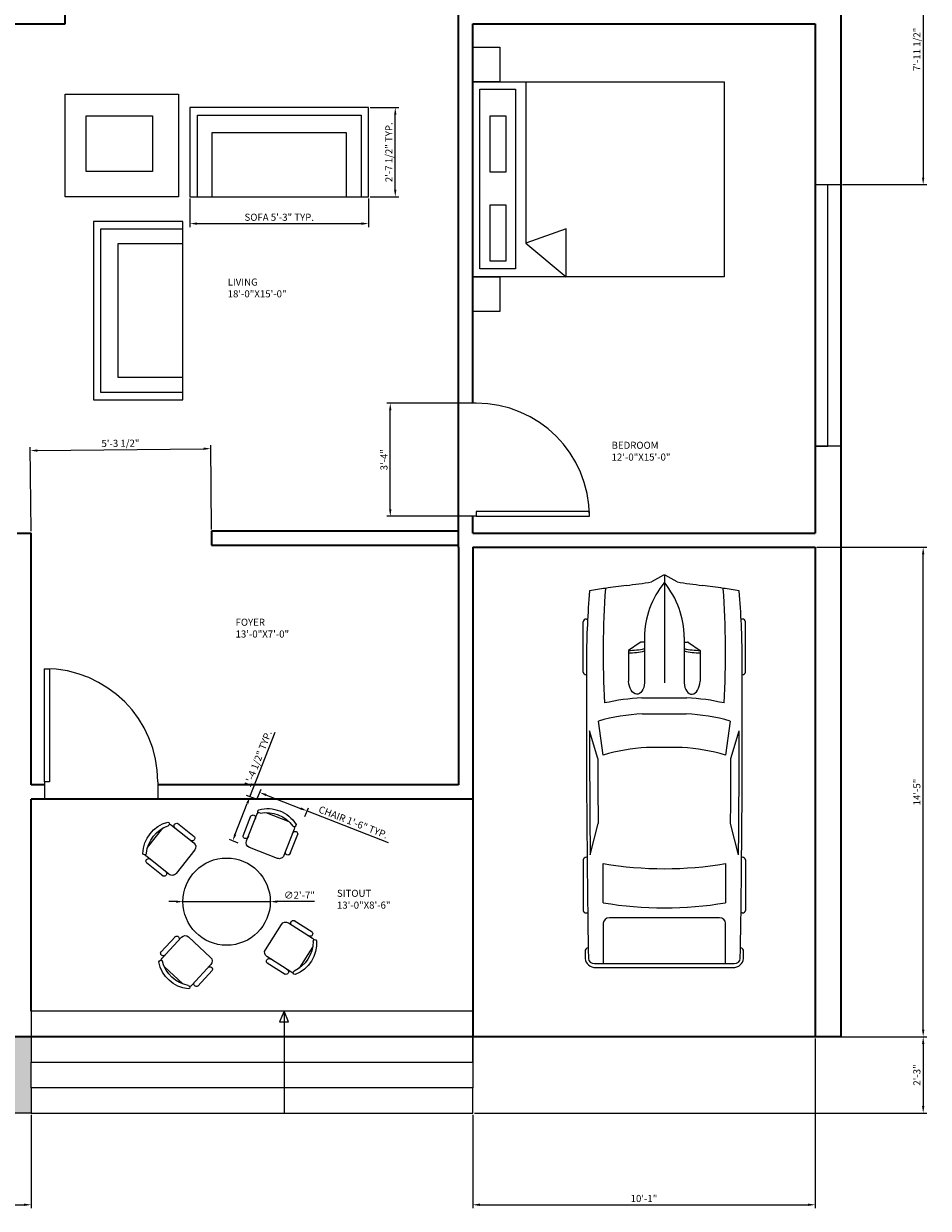
# Model space of a CAD drawing. Units: inches. Extents: x 2981 to 3526, y 1512 to 2158.
# Tile 3 of 4: x 3207 to 3526, y 1512 to 1930. Entities that reach past the tile are written whole.
import ezdxf

# ---------------------------------------------------------------- set-up
doc = ezdxf.new("R2010")
doc.units = ezdxf.units.IN
for name, color, linetype, lineweight in [('A-ANNO-DIMS', 2, 'Continuous', 18), ('A-AREA-IDEN', 7, 'Continuous', 18), ('A-DOOR', 4, 'Continuous', 25), ('A-FLOR-STRS', 7, 'Continuous', 25), ('A-FURN', 8, 'Continuous', 18), ('A-GLAZ', 4, 'Continuous', 18), ('A-WALL', 7, 'Continuous', 35), ('C-PKNG-VEHI', 8, 'Continuous', 13), ('L-GRND-PATT', 8, 'Continuous', 13), ('L-PLNT-BEDS', 7, 'Continuous', 18)]:
    doc.layers.add(name, color=color, linetype=linetype, lineweight=lineweight)
doc.styles.get("Standard").update_dxf_attribs({"font": 'arial.ttf'})
doc.dimstyles.new('ISO-25', dxfattribs={"dimtxt": 2.5, "dimasz": 2.5, "dimexe": 1.25, "dimexo": 0.625, "dimtad": 1, "dimlunit": 3, "dimtxsty": 'Standard', "dimcen": 2.5, "dimadec": 0, "dimazin": 0, "dimtfac": 1, "dimtmove": 0, "dimatfit": 3, "dimfxl": 1, "dimarcsym": 0})

# ---------------------------------------------------------------- blocks, each defined once
blk = doc.blocks.new('*U2')
for p, q in [((0, 0), (0, -6)), ((40, 0), (40, -6))]:
    blk.add_line(p, q)
blk.add_lwpolyline([(0, 0), (0, 40), (1.75, 40), (1.75, 0)], close=True)
blk.add_arc((0, 0), 40, 0, 90)
blk = doc.blocks.new('*U3')
for p, q in [((0, 0), (0, -6)), ((-40, 0), (-40, -6))]:
    blk.add_line(p, q)
blk.add_lwpolyline([(0, 0), (0, 40), (-1.75, 40), (-1.75, 0)], close=True)
blk.add_arc((0, 0), 40, 90, 180)
blk = doc.blocks.new('*U7')
for p, q in [((21.1, 37.41), (21.1, 36.83)), ((46.55, 38.89), (22.35, 38.89)), ((47.8, 37.39), (47.8, 37.41)), ((87.99, 31.87), (74.76, 35.92)), ((134.31, 35.6), (119.29, 31.78)), ((135.45, 37.07), (135.45, 37.41)), ((136.7, 38.89), (160.9, 38.89)), ((162.15, 37.41), (162.15, 36.77)), ((70.03, 31.54), (86.41, 29.35)), ((138.42, 29.35), (157.25, 29.35)), ((186.47, 29.35), (167.01, 29.35)), ((186.47, -33.5), (186.47, 33.5)), ((188.4, -32.76), (188.4, 32.76)), ((164.52, 26.39), (164.52, -26.39)), ((32.27, 11.63), (36.13, 17.17)), ((36.13, 17.17), (50.94, 17.17)), ((3.27, 6.13), (0.1, 0.41)), ((29.77, 9.51), (51.68, 9.51)), ((32.12, 9.51), (32.12, 11.15)), ((58.92, -10.77), (58.92, 10.77)), ((66.55, -10.53), (66.55, 10.53)), ((82.74, 8.5), (82.74, -8.5)), ((186.47, -10.53), (186.47, 10.53)), ((0, 0), (51.68, 0)), ((0.1, -0.41), (3.27, -6.13)), ((29.77, -9.51), (51.68, -9.51)), ((32.12, -9.51), (32.12, -11.15)), ((32.27, -11.63), (36.13, -17.17)), ((36.13, -17.17), (50.94, -17.17)), ((86.41, -29.35), (70.03, -31.54)), ((87.99, -31.87), (74.76, -35.92)), ((134.31, -35.6), (119.29, -31.78)), ((157.25, -29.35), (138.42, -29.35)), ((167.01, -29.35), (186.47, -29.35)), ((21.1, -37.41), (21.1, -36.83)), ((46.55, -38.89), (22.35, -38.89)), ((47.8, -37.39), (47.8, -37.41)), ((135.45, -37.07), (135.45, -37.41)), ((136.7, -38.89), (160.9, -38.89)), ((162.15, -37.41), (162.15, -36.77))]:
    blk.add_line(p, q)
for centre, major_axis, ratio, start_param, end_param in [((266.03, -27.52), (0, 313.31), 0.842304, 1.367076, 1.39176), ((41.19, -490.86), (0, 528.23), 0.842304, 0.00281, 0.075598), ((22.35, 37.41), (0, -1.48), 0.842304, 3.141593, 4.712389), ((64.48, -10555.62), (0, 10593.03), 0.842304, -0.013397, 0.002797), ((46.55, 37.41), (0, 1.48), 0.842304, -1.570796, 0), ((64.48, -10555.62), (0, -10591.55), 0.842304, 3.133765, 3.140441), ((136.7, 37.41), (0, -1.48), 0.842304, 3.141593, 4.712389), ((160.9, 37.41), (0, 1.48), 0.842304, -1.570796, 0), ((180.63, 35.84), (0, 2.22), 0.842304, -0.013017, 1.249894), ((64.48, -10556.36), (0, 10595.31), 0.842304, -0.013397, -0.013017), ((183.98, 33.5), (0, -2.96), 0.842304, 1.570796, 3.128196), ((183.98, 32.76), (0, -5.25), 0.842304, 1.570796, 3.128196), ((37.47, -593.96), (0, -623.33), 0.842304, 3.096046, 3.200911), ((134.4, 5.39), (0, -89.78), 0.842304, 4.449482, 4.652344), ((135.29, 5.39), (0, 81.77), 0.842304, 1.245306, 1.50788), ((149.6, 2.8), (0, -79.58), 0.842304, 4.372215, 4.640744), ((95.79, -3666.35), (0, -3698.24), 0.842304, 3.134049, 3.144098), ((17.08, 0), (0, 147.02), 0.842304, 4.511394, 4.913384), ((35.91, 0), (0, 147.02), 0.842304, 4.511394, 4.913384), ((167.01, 26.39), (0, 2.96), 0.842304, 0, 1.570796), ((259.18, -27.52), (0, -305.3), 0.842304, 4.528606, 4.561838), ((-204.49, 52.4), (0, -250.96), 0.842304, 1.385369, 1.434372), ((13.04, 17.01), (0, 27.42), 0.842304, 4.435146, 4.718221), ((14.2, 17.01), (0, 27.42), 0.842304, 4.435146, 4.718221), ((50.79, 13.34), (6.34, -0.36), 0.603834, -1.395552, 1.581315), ((32.75, 11.15), (0, 0.74), 0.842304, 0.879714, 1.570796), ((29.77, -46.66), (0, 56.17), 0.842304, 0, 0.590319), ((0.62, 0), (0, -0.74), 0.842304, 4.131459, 5.293319), ((29.77, 46.66), (0, 56.17), 0.842304, 2.551274, 3.141593), ((-204.49, -52.4), (0, 250.96), 0.842304, -1.434372, -1.385369), ((32.75, -11.15), (0, -0.74), 0.842304, 4.712389, 5.403472), ((13.04, -17.01), (0, -27.42), 0.842304, 1.564964, 1.848039), ((14.2, -17.01), (0, -27.42), 0.842304, 1.564964, 1.848039), ((134.4, -5.39), (0, -89.78), 0.842304, -1.510751, -1.307889), ((135.29, -5.39), (0, -81.77), 0.842304, -1.50788, -1.245306), ((149.6, -2.8), (0, -79.58), 0.842304, -1.499151, -1.230623), ((259.18, 27.52), (0, 305.3), 0.842304, 1.721348, 1.754579), ((266.03, 27.52), (0, 313.31), 0.842304, 1.749832, 1.774517), ((37.47, 593.96), (0, -623.33), 0.842304, -0.059319, 0.045547), ((167.01, -26.39), (0, -2.96), 0.842304, 4.712389, 6.283185), ((95.79, 3666.35), (0, -3698.24), 0.842304, -0.002505, 0.007544), ((183.98, -33.5), (0, 2.96), 0.842304, 3.15499, 4.712389), ((183.98, -32.76), (0, -5.25), 0.842304, 0.013397, 1.570796), ((41.19, 490.86), (0, -528.23), 0.842304, -0.075598, -0.00281), ((22.35, -37.41), (0, 1.48), 0.842304, 1.570796, 3.141593), ((64.48, 10555.62), (0, 10593.03), 0.842304, 3.138796, 3.15499), ((46.55, -37.41), (0, -1.48), 0.842304, 0, 1.570796), ((64.48, 10555.62), (0, -10591.55), 0.842304, 0.001152, 0.007828), ((136.7, -37.41), (0, -1.48), 0.842304, -1.570796, 0), ((160.9, -37.41), (0, 1.48), 0.842304, 3.141593, 4.712389), ((180.63, -35.84), (0, -2.22), 0.842304, -1.249894, 0.013017), ((64.48, 10556.36), (0, 10595.31), 0.842304, 3.15461, 3.15499)]:
    blk.add_ellipse(centre, major_axis=major_axis, ratio=ratio, start_param=start_param, end_param=end_param)
at = {"extrusion": (0, 0, -1)}
blk.add_ellipse((50.79, -13.34), major_axis=(6.34, 0.36), ratio=0.603834, start_param=-1.395552, end_param=1.581315, dxfattribs=at)
blk = doc.blocks.new('SOFA2')
for p, q in [((-36, 0), (-36, -36)), ((36, 0), (-36, 0)), ((36, -36), (36, 0)), ((-33, -36), (-33, -3)), ((-33, -3), (33, -3)), ((33, -3), (33, -36)), ((-27, -36), (-27, -10)), ((-27, -10), (27, -10)), ((27, -10), (27, -36)), ((-36, -36), (36, -36))]:
    blk.add_line(p, q)
blk = doc.blocks.new('CHAIR7')
for p, q in [((5.12, 15.04), (17.88, 15.04)), ((0, 9), (0, -9)), ((20, 12), (3, 12)), ((23, -7.44), (23, 7.44)), ((3, -12), (20, -12)), ((5.12, -15), (17.88, -15))]:
    blk.add_line(p, q)
for centre, radius, start, end in [((5.56, 13.54), 1.56, 73.7398, 286.2602), ((17.44, 13.54), 1.56, 253.7398, 106.2602), ((3, 9), 3, 90, 180), ((20, 9), 3, 62.41556, 90), ((22.34, 11.12), 1.1, 53.30994, 212.02741), ((4.82, 0), 19.64, 327.57575, 32.42425), ((7, 0), 20, 323.1301, 36.8699), ((3, -9), 3, 180, 270), ((5.56, -13.5), 1.56, 73.7398, 286.2602), ((17.44, -13.5), 1.56, 253.7398, 106.2602), ((20, -9), 3, 270, 297.58444), ((22.34, -11.12), 1.1, 147.97259, 306.69006)]:
    blk.add_arc(centre, radius, start, end)
blk = doc.blocks.new('WIN-92IN-BEDROOM')
for p, q in [((0, 92.47), (9, 92.47)), ((0, 92.47), (0, 0)), ((4.5, 0), (4.5, 92.47)), ((9, 92.47), (9, 0)), ((9, 0), (0, 0)), ((0, 0), (4.5, 0))]:
    blk.add_line(p, q)
blk = doc.blocks.new('BED-DOUBLE-WITH-NIGHTSTANDS')
for p, q in [((18.84, 81.09), (18.84, 24.12)), ((33.02, 29.21), (18.84, 24.12)), ((33.02, 12.24), (33.02, 29.21)), ((18.84, 24.12), (33.02, 12.24))]:
    blk.add_line(p, q)
for points in [[(9.63, 93.35), (9.63, 81.1), (0.08, 81.1), (0.08, 93.35)], [(0.08, 12.24), (0.08, 81.09), (88.86, 81.09), (88.86, 12.24)], [(2.5, 15.01), (2.5, 78.54), (15.13, 78.54), (15.13, 15.01)], [(6.2, 49.25), (6.2, 69.14), (11.74, 69.14), (11.74, 49.25)], [(6.2, 17.79), (6.2, 37.68), (11.74, 37.68), (11.74, 17.79)], [(9.63, 12.24), (9.63, 0), (0, 0), (0, 12.24)]]:
    blk.add_lwpolyline(points, close=True)
blk = doc.blocks.new('*D23')
at = {"layer": 'A-ANNO-DIMS', "color": 0, "lineweight": -2, "transparency": 16777216}
for p, q in [((3289.4, 1656.6), (3290.6, 1659.7)), ((3292.48, 1657.62), (3304.54, 1652.91)), ((3306.12, 1650.08), (3307.32, 1653.17)), ((3306.87, 1652), (3335.56, 1640.81))]:
    blk.add_line(p, q, dxfattribs=at)
at = {"layer": 'A-ANNO-DIMS', "color": 0, "transparency": 16777216}
for points in [[(3292.63, 1658.01), (3292.33, 1657.23), (3290.15, 1658.53)], [(3304.69, 1653.3), (3304.39, 1652.53), (3306.87, 1652)]]:
    blk.add_solid(points, dxfattribs=at)
at = {"layer": 'Defpoints', "color": 0, "transparency": 16777216}
for p in [(3289.17, 1656.02), (3305.89, 1649.5), (3306.87, 1652)]:
    blk.add_point(p, dxfattribs=at)
at = {"layer": 'A-ANNO-DIMS', "color": 0, "transparency": 16777216, "insert": (3323.08, 1647.74), "char_height": 2.5, "attachment_point": 5, "rotation": 338.6778}
blk.add_mtext('CHAIR 1\'-6" TYP.', dxfattribs=at)
blk = doc.blocks.new('*D24')
at = {"layer": 'A-ANNO-DIMS', "color": 0, "lineweight": -2, "transparency": 16777216}
for p, q in [((3286.66, 1657), (3295.6, 1679.9)), ((3281.49, 1643.75), (3285.75, 1654.67)), ((3288.59, 1656.25), (3285.5, 1657.46)), ((3282.51, 1640.67), (3279.42, 1641.88))]:
    blk.add_line(p, q, dxfattribs=at)
at = {"layer": 'A-ANNO-DIMS', "color": 0, "transparency": 16777216}
for points in [[(3285.37, 1654.82), (3286.14, 1654.52), (3286.66, 1657)], [(3281.1, 1643.91), (3281.88, 1643.6), (3280.58, 1641.43)]]:
    blk.add_solid(points, dxfattribs=at)
at = {"layer": 'Defpoints', "color": 0, "transparency": 16777216}
for p in [(3286.66, 1657), (3289.17, 1656.02), (3283.09, 1640.45)]:
    blk.add_point(p, dxfattribs=at)
at = {"layer": 'A-ANNO-DIMS', "color": 0, "transparency": 16777216, "insert": (3289.8, 1670.31), "char_height": 2.5, "attachment_point": 5, "rotation": 68.6778}
blk.add_mtext('1\'-4 1/2" TYP.', dxfattribs=at)
blk = doc.blocks.new('*D25')
at = {"layer": 'A-ANNO-DIMS', "color": 0, "lineweight": -2, "transparency": 16777216}
for p, q in [((3265.49, 1868.39), (3265.49, 1858.31)), ((3328.56, 1868.39), (3328.56, 1858.31)), ((3267.99, 1859.56), (3326.06, 1859.56))]:
    blk.add_line(p, q, dxfattribs=at)
at = {"layer": 'A-ANNO-DIMS', "color": 0, "transparency": 16777216}
for points in [[(3267.99, 1859.98), (3267.99, 1859.14), (3265.49, 1859.56)], [(3326.06, 1859.98), (3326.06, 1859.14), (3328.56, 1859.56)]]:
    blk.add_solid(points, dxfattribs=at)
at = {"layer": 'Defpoints', "color": 0, "transparency": 16777216}
for p in [(3265.49, 1869.02), (3328.56, 1869.02), (3328.56, 1859.56)]:
    blk.add_point(p, dxfattribs=at)
at = {"layer": 'A-ANNO-DIMS', "color": 0, "transparency": 16777216, "insert": (3297.03, 1861.48), "char_height": 2.5, "attachment_point": 5}
blk.add_mtext('SOFA 5\'-3" TYP.', dxfattribs=at)
blk = doc.blocks.new('*D26')
at = {"layer": 'A-ANNO-DIMS', "color": 0, "lineweight": -2, "transparency": 16777216}
for p, q in [((3329.19, 1900.55), (3339.27, 1900.55)), ((3338.02, 1871.52), (3338.02, 1898.05)), ((3329.19, 1869.02), (3339.27, 1869.02))]:
    blk.add_line(p, q, dxfattribs=at)
at = {"layer": 'A-ANNO-DIMS', "color": 0, "transparency": 16777216}
for points in [[(3337.6, 1898.05), (3338.44, 1898.05), (3338.02, 1900.55)], [(3337.6, 1871.52), (3338.44, 1871.52), (3338.02, 1869.02)]]:
    blk.add_solid(points, dxfattribs=at)
at = {"layer": 'Defpoints', "color": 0, "transparency": 16777216}
for p in [(3328.56, 1900.55), (3338.02, 1900.55), (3328.56, 1869.02)]:
    blk.add_point(p, dxfattribs=at)
at = {"layer": 'A-ANNO-DIMS', "color": 0, "transparency": 16777216, "insert": (3336.1, 1884.79), "char_height": 2.5, "attachment_point": 5, "rotation": 90}
blk.add_mtext('2\'-7 1/2" TYP.', dxfattribs=at)
blk = doc.blocks.new('*D35')
at = {"layer": 'A-ANNO-DIMS', "color": 0, "lineweight": -2, "transparency": 16777216}
for p, q in [((3364.77, 1796.13), (3335, 1796.13)), ((3336.25, 1758.63), (3336.25, 1793.63)), ((3364.77, 1756.13), (3335, 1756.13))]:
    blk.add_line(p, q, dxfattribs=at)
at = {"layer": 'A-ANNO-DIMS', "color": 0, "transparency": 16777216}
for points in [[(3335.84, 1793.63), (3336.67, 1793.63), (3336.25, 1796.13)], [(3335.84, 1758.63), (3336.67, 1758.63), (3336.25, 1756.13)]]:
    blk.add_solid(points, dxfattribs=at)
at = {"layer": 'Defpoints', "color": 0, "transparency": 16777216}
for p in [(3336.25, 1796.13), (3365.4, 1796.13), (3365.4, 1756.13)]:
    blk.add_point(p, dxfattribs=at)
at = {"layer": 'A-ANNO-DIMS', "color": 0, "transparency": 16777216, "insert": (3334.35, 1776.13), "char_height": 2.5, "attachment_point": 5, "rotation": 90}
blk.add_mtext('3\'-4"', dxfattribs=at)
blk = doc.blocks.new('*D37')
at = {"layer": 'A-ANNO-DIMS', "color": 0, "lineweight": -2, "transparency": 16777216}
for p, q in [((3496.02, 1572.2), (3525.79, 1572.2)), ((3524.54, 1569.7), (3524.54, 1547.7)), ((3366.02, 1545.2), (3525.79, 1545.2))]:
    blk.add_line(p, q, dxfattribs=at)
at = {"layer": 'A-ANNO-DIMS', "color": 0, "transparency": 16777216}
for points in [[(3524.13, 1569.7), (3524.96, 1569.7), (3524.54, 1572.2)], [(3524.13, 1547.7), (3524.96, 1547.7), (3524.54, 1545.2)]]:
    blk.add_solid(points, dxfattribs=at)
at = {"layer": 'Defpoints', "color": 0, "transparency": 16777216}
for p in [(3495.4, 1572.2), (3365.4, 1545.2), (3524.54, 1545.2)]:
    blk.add_point(p, dxfattribs=at)
at = {"layer": 'A-ANNO-DIMS', "color": 0, "transparency": 16777216, "insert": (3522.64, 1558.7), "char_height": 2.5, "attachment_point": 5, "rotation": 90}
blk.add_mtext('2\'-3"', dxfattribs=at)
blk = doc.blocks.new('*D38')
at = {"layer": 'A-ANNO-DIMS', "color": 0, "lineweight": -2, "transparency": 16777216}
for p, q in [((3486.4, 1571.58), (3486.4, 1511.59)), ((3365.4, 1544.58), (3365.4, 1511.59)), ((3367.9, 1512.84), (3483.9, 1512.84))]:
    blk.add_line(p, q, dxfattribs=at)
at = {"layer": 'A-ANNO-DIMS', "color": 0, "transparency": 16777216}
for points in [[(3367.9, 1513.26), (3367.9, 1512.43), (3365.4, 1512.84)], [(3483.9, 1513.26), (3483.9, 1512.43), (3486.4, 1512.84)]]:
    blk.add_solid(points, dxfattribs=at)
at = {"layer": 'Defpoints', "color": 0, "transparency": 16777216}
for p in [(3486.4, 1572.2), (3365.4, 1545.2), (3486.4, 1512.84)]:
    blk.add_point(p, dxfattribs=at)
at = {"layer": 'A-ANNO-DIMS', "color": 0, "transparency": 16777216, "insert": (3425.9, 1514.75), "char_height": 2.5, "attachment_point": 5}
blk.add_mtext('10\'-1"', dxfattribs=at)
blk = doc.blocks.new('*D39')
at = {"layer": 'A-ANNO-DIMS', "color": 0, "lineweight": -2, "transparency": 16777216}
for p, q in [((3487.02, 1745.2), (3525.79, 1745.2)), ((3524.54, 1574.7), (3524.54, 1742.7)), ((3487.02, 1572.2), (3525.79, 1572.2))]:
    blk.add_line(p, q, dxfattribs=at)
at = {"layer": 'A-ANNO-DIMS', "color": 0, "transparency": 16777216}
for points in [[(3524.13, 1742.7), (3524.96, 1742.7), (3524.54, 1745.2)], [(3524.13, 1574.7), (3524.96, 1574.7), (3524.54, 1572.2)]]:
    blk.add_solid(points, dxfattribs=at)
at = {"layer": 'Defpoints', "color": 0, "transparency": 16777216}
for p in [(3486.4, 1745.2), (3524.54, 1745.2), (3486.4, 1572.2)]:
    blk.add_point(p, dxfattribs=at)
at = {"layer": 'A-ANNO-DIMS', "color": 0, "transparency": 16777216, "insert": (3522.64, 1658.7), "char_height": 2.5, "attachment_point": 5, "rotation": 90}
blk.add_mtext('14\'-5"', dxfattribs=at)
blk = doc.blocks.new('*D40')
at = {"layer": 'A-ANNO-DIMS', "color": 0, "lineweight": -2, "transparency": 16777216}
for p, q in [((3015.4, 1544.58), (3015.4, 1511.59)), ((3209.4, 1544.58), (3209.4, 1511.59)), ((3017.9, 1512.84), (3206.9, 1512.84))]:
    blk.add_line(p, q, dxfattribs=at)
at = {"layer": 'A-ANNO-DIMS', "color": 0, "transparency": 16777216}
for points in [[(3017.9, 1513.26), (3017.9, 1512.43), (3015.4, 1512.84)], [(3206.9, 1513.26), (3206.9, 1512.43), (3209.4, 1512.84)]]:
    blk.add_solid(points, dxfattribs=at)
at = {"layer": 'Defpoints', "color": 0, "transparency": 16777216}
for p in [(3015.4, 1545.2), (3209.4, 1545.2), (3209.4, 1512.84)]:
    blk.add_point(p, dxfattribs=at)
at = {"layer": 'A-ANNO-DIMS', "color": 0, "transparency": 16777216, "insert": (3112.4, 1514.75), "char_height": 2.5, "attachment_point": 5}
blk.add_mtext('16\'-2"', dxfattribs=at)
blk = doc.blocks.new('*D42')
at = {"layer": 'A-ANNO-DIMS', "color": 0, "lineweight": -2, "transparency": 16777216}
for p, q in [((3496.02, 1968.93), (3525.79, 1968.93)), ((3524.54, 1966.43), (3524.54, 1875.83)), ((3496.02, 1873.33), (3525.79, 1873.33))]:
    blk.add_line(p, q, dxfattribs=at)
at = {"layer": 'A-ANNO-DIMS', "color": 0, "transparency": 16777216}
for points in [[(3524.13, 1966.43), (3524.96, 1966.43), (3524.54, 1968.93)], [(3524.13, 1875.83), (3524.96, 1875.83), (3524.54, 1873.33)]]:
    blk.add_solid(points, dxfattribs=at)
at = {"layer": 'Defpoints', "color": 0, "transparency": 16777216}
for p in [(3495.4, 1968.93), (3495.4, 1873.33), (3524.54, 1873.33)]:
    blk.add_point(p, dxfattribs=at)
at = {"layer": 'A-ANNO-DIMS', "color": 0, "transparency": 16777216, "insert": (3522.63, 1921.13), "char_height": 2.5, "attachment_point": 5, "rotation": 90}
blk.add_mtext('7\'-11 1/2"', dxfattribs=at)
blk = doc.blocks.new('*D56')
at = {"layer": 'A-ANNO-DIMS', "color": 0, "lineweight": -2, "transparency": 16777216}
for p, q in [((3209.39, 1750.83), (3209.07, 1780.6)), ((3211.58, 1779.37), (3270.32, 1780.01)), ((3273.13, 1751.52), (3272.81, 1781.29))]:
    blk.add_line(p, q, dxfattribs=at)
at = {"layer": 'A-ANNO-DIMS', "color": 0, "transparency": 16777216}
for points in [[(3211.58, 1779.79), (3211.59, 1778.96), (3209.08, 1779.35)], [(3270.32, 1780.43), (3270.33, 1779.59), (3272.82, 1780.04)]]:
    blk.add_solid(points, dxfattribs=at)
at = {"layer": 'Defpoints', "color": 0, "transparency": 16777216}
for p in [(3272.82, 1780.04), (3209.4, 1750.2), (3273.14, 1750.89)]:
    blk.add_point(p, dxfattribs=at)
at = {"layer": 'A-ANNO-DIMS', "color": 0, "transparency": 16777216, "insert": (3240.93, 1781.61), "char_height": 2.5, "attachment_point": 5, "rotation": 0.6207}
blk.add_mtext('5\'-3 1/2"', dxfattribs=at)
blk = doc.blocks.new('*D57')
at = {"layer": 'A-ANNO-DIMS', "color": 0, "lineweight": -2, "transparency": 16777216}
for p, q in [((3260.51, 1619.96), (3258.01, 1619.96)), ((3263.01, 1619.96), (3293.85, 1619.96)), ((3309.46, 1619.96), (3296.35, 1619.96))]:
    blk.add_line(p, q, dxfattribs=at)
at = {"layer": 'A-ANNO-DIMS', "color": 0, "transparency": 16777216}
for points in [[(3260.51, 1620.38), (3260.51, 1619.54), (3263.01, 1619.96)], [(3296.35, 1620.38), (3296.35, 1619.54), (3293.85, 1619.96)]]:
    blk.add_solid(points, dxfattribs=at)
at = {"layer": 'Defpoints', "color": 0, "transparency": 16777216}
for p in [(3263.01, 1619.96), (3293.85, 1619.96)]:
    blk.add_point(p, dxfattribs=at)
at = {"layer": 'A-ANNO-DIMS', "color": 0, "transparency": 16777216, "insert": (3304.15, 1621.93), "char_height": 2.5, "attachment_point": 5, "rotation": 0.0008}
blk.add_mtext('∅2\'-7"', dxfattribs=at)

msp = doc.modelspace()

# ---------------------------------------------------------------- hatches: boundary and pattern name
at = {"layer": 'L-GRND-PATT'}
h = msp.add_hatch(color=256, dxfattribs=at)
h.dxf.hatch_style = 1
h.paths.add_polyline_path([(3209.399, 1563.202), (3209.399, 1572.202), (3015.399, 1572.202), (3015.399, 1545.202), (3209.399, 1545.202), (3209.399, 1554.202)])
h.paths.add_polyline_path([(3038.736, 1554.203), (3037.324, 1553.709), (3036.297, 1553.792), (3035.398, 1554.532), (3035.27, 1554.121), (3035.719, 1553.627), (3034.371, 1553.956), (3032.573, 1553.956), (3033.344, 1553.545), (3032.638, 1553.462), (3031.867, 1553.709), (3030.968, 1553.627), (3031.418, 1553.298), (3030.327, 1553.545), (3030.968, 1553.133), (3028.914, 1553.627), (3028.722, 1554.039), (3027.759, 1553.462), (3027.566, 1554.039), (3026.668, 1553.462), (3026.411, 1553.956), (3026.09, 1554.203), (3025.512, 1553.956), (3025.384, 1553.709), (3024.677, 1554.039), (3024.549, 1554.779), (3024.164, 1554.368), (3023.073, 1554.039), (3022.623, 1554.039), (3022.559, 1554.45), (3022.752, 1554.861), (3022.11, 1554.779), (3021.532, 1554.45), (3021.532, 1555.108), (3020.697, 1554.944), (3021.147, 1555.684), (3020.505, 1555.602), (3020.376, 1555.849), (3019.991, 1556.096), (3019.927, 1556.59), (3020.569, 1556.178), (3021.403, 1556.178), (3022.302, 1556.343), (3022.816, 1556.837), (3022.944, 1556.507), (3023.458, 1557.413), (3024.613, 1557.577), (3025.319, 1558.483), (3025.512, 1559.306), (3024.742, 1559.635), (3024.934, 1559.882), (3025.384, 1559.882), (3024.292, 1560.458), (3023.971, 1559.964), (3022.944, 1559.799), (3022.559, 1560.293), (3021.853, 1560.211), (3021.724, 1560.046), (3021.211, 1560.293), (3021.468, 1560.622), (3022.366, 1560.869), (3023.907, 1561.528), (3024.613, 1562.433), (3024.677, 1562.927), (3026.346, 1563.832), (3026.732, 1564.408), (3026.282, 1564.408), (3026.539, 1564.82), (3026.09, 1564.82), (3025.539, 1564.994), (3024.913, 1564.765), (3024.485, 1564.984), (3023.907, 1564.82), (3023.586, 1564.655), (3023.907, 1565.149), (3024.806, 1565.807), (3025.961, 1566.301), (3026.86, 1566.877), (3026.924, 1567.042), (3026.411, 1566.959), (3026.603, 1567.124), (3027.245, 1567.535), (3027.695, 1568.194), (3027.502, 1568.77), (3027.117, 1568.852), (3026.732, 1568.688), (3027.117, 1569.181), (3028.08, 1569.511), (3028.657, 1570.004), (3029.031, 1571.432), (3029.416, 1569.95), (3029.898, 1569.332), (3030.778, 1568.968), (3030.466, 1568.968), (3030.126, 1568.786), (3030.154, 1568.604), (3030.636, 1568.059), (3031.771, 1567.804), (3031.005, 1567.695), (3030.324, 1567.44), (3030.523, 1567.368), (3030.381, 1567.113), (3030.977, 1567.258), (3030.494, 1566.895), (3031.175, 1566.713), (3030.92, 1566.604), (3031.459, 1565.949), (3032.566, 1565.767), (3033.133, 1566.131), (3033.417, 1566.494), (3033.389, 1566.313), (3033.332, 1565.803), (3032.878, 1565.294), (3032.736, 1564.712), (3032.254, 1564.712), (3032.793, 1564.457), (3033.445, 1564.348), (3033.956, 1564.494), (3033.559, 1564.203), (3032.935, 1564.057), (3033.247, 1563.985), (3032.651, 1563.693), (3032.991, 1563.621), (3031.941, 1563.439), (3032.566, 1562.966), (3033.559, 1562.748), (3034.609, 1562.857), (3035.034, 1563.184), (3035.063, 1562.857), (3035.808, 1562.379), (3035.27, 1561.775), (3034.949, 1561.034), (3033.472, 1560.869), (3032.638, 1560.458), (3033.28, 1559.882), (3033.857, 1560.046), (3034.114, 1559.47), (3034.499, 1559.635), (3034.949, 1559.059), (3036.233, 1558.894), (3037.131, 1559.059), (3037.388, 1558.4), (3036.746, 1558.483), (3035.783, 1558.153), (3036.104, 1557.495), (3034.884, 1557.495), (3033.408, 1556.507), (3034.307, 1556.014), (3034.884, 1556.014), (3035.591, 1556.014), (3036.104, 1555.52), (3036.489, 1555.438), (3036.618, 1555.767), (3037.003, 1555.191), (3037.388, 1555.191), (3037.388, 1554.697), (3037.837, 1554.697), (3037.837, 1554.368), (3038.415, 1554.45)], flags=16)
h.paths.add_polyline_path([(3069.74, 1556.59), (3070.382, 1556.178), (3071.217, 1556.178), (3072.115, 1556.343), (3072.629, 1556.837), (3072.757, 1556.507), (3073.271, 1557.413), (3074.426, 1557.577), (3075.133, 1558.483), (3075.325, 1559.306), (3074.555, 1559.635), (3074.747, 1559.882), (3075.197, 1559.882), (3074.105, 1560.458), (3073.785, 1559.964), (3072.757, 1559.799), (3072.372, 1560.293), (3071.666, 1560.211), (3071.538, 1560.046), (3071.024, 1560.293), (3071.281, 1560.622), (3072.18, 1560.869), (3073.72, 1561.528), (3074.426, 1562.433), (3074.491, 1562.927), (3076.16, 1563.832), (3076.545, 1564.408), (3076.096, 1564.408), (3076.352, 1564.82), (3075.903, 1564.82), (3075.352, 1564.994), (3074.726, 1564.765), (3074.298, 1564.984), (3073.72, 1564.82), (3073.399, 1564.655), (3073.72, 1565.149), (3074.619, 1565.807), (3075.774, 1566.301), (3076.673, 1566.877), (3076.737, 1567.042), (3076.224, 1566.959), (3076.416, 1567.124), (3077.058, 1567.535), (3077.508, 1568.194), (3077.315, 1568.77), (3076.93, 1568.852), (3076.545, 1568.688), (3076.93, 1569.181), (3077.893, 1569.511), (3078.471, 1570.004), (3078.844, 1571.432), (3079.229, 1569.95), (3079.712, 1569.332), (3080.591, 1568.968), (3080.279, 1568.968), (3079.939, 1568.786), (3079.967, 1568.604), (3080.449, 1568.059), (3081.584, 1567.804), (3080.818, 1567.695), (3080.137, 1567.44), (3080.336, 1567.368), (3080.194, 1567.113), (3080.79, 1567.258), (3080.308, 1566.895), (3080.989, 1566.713), (3080.733, 1566.604), (3081.272, 1565.949), (3082.379, 1565.767), (3082.946, 1566.131), (3083.23, 1566.494), (3083.202, 1566.313), (3083.145, 1565.803), (3082.691, 1565.294), (3082.549, 1564.712), (3082.067, 1564.712), (3082.606, 1564.457), (3083.258, 1564.348), (3083.769, 1564.494), (3083.372, 1564.203), (3082.748, 1564.057), (3083.06, 1563.985), (3082.464, 1563.693), (3082.804, 1563.621), (3081.755, 1563.439), (3082.379, 1562.966), (3083.372, 1562.748), (3084.422, 1562.857), (3084.847, 1563.184), (3084.876, 1562.857), (3085.622, 1562.379), (3085.083, 1561.775), (3084.762, 1561.034), (3083.285, 1560.869), (3082.451, 1560.458), (3083.093, 1559.882), (3083.67, 1560.046), (3083.927, 1559.47), (3084.312, 1559.635), (3084.762, 1559.059), (3086.046, 1558.894), (3086.945, 1559.059), (3087.201, 1558.4), (3086.559, 1558.483), (3085.596, 1558.153), (3085.917, 1557.495), (3084.698, 1557.495), (3083.221, 1556.507), (3084.12, 1556.014), (3084.698, 1556.014), (3085.404, 1556.014), (3085.917, 1555.52), (3086.303, 1555.438), (3086.431, 1555.767), (3086.816, 1555.191), (3087.201, 1555.191), (3087.201, 1554.697), (3087.651, 1554.697), (3087.651, 1554.368), (3088.228, 1554.45), (3088.549, 1554.203), (3087.137, 1553.709), (3086.11, 1553.792), (3085.211, 1554.532), (3085.083, 1554.121), (3085.532, 1553.627), (3084.184, 1553.956), (3082.387, 1553.956), (3083.157, 1553.545), (3082.451, 1553.462), (3081.68, 1553.709), (3080.782, 1553.627), (3081.231, 1553.298), (3080.14, 1553.545), (3080.782, 1553.133), (3078.728, 1553.627), (3078.535, 1554.039), (3077.572, 1553.462), (3077.379, 1554.039), (3076.481, 1553.462), (3076.224, 1553.956), (3075.903, 1554.203), (3075.325, 1553.956), (3075.197, 1553.709), (3074.491, 1554.039), (3074.362, 1554.779), (3073.977, 1554.368), (3072.886, 1554.039), (3072.436, 1554.039), (3072.372, 1554.45), (3072.565, 1554.861), (3071.923, 1554.779), (3071.345, 1554.45), (3071.345, 1555.108), (3070.51, 1554.944), (3070.96, 1555.684), (3070.318, 1555.602), (3070.19, 1555.849), (3069.804, 1556.096)], flags=16)
h.paths.add_polyline_path([(3120.884, 1556.59), (3121.526, 1556.178), (3122.361, 1556.178), (3123.259, 1556.343), (3123.773, 1556.837), (3123.901, 1556.507), (3124.415, 1557.413), (3125.57, 1557.577), (3126.277, 1558.483), (3126.469, 1559.306), (3125.699, 1559.635), (3125.891, 1559.882), (3126.341, 1559.882), (3125.249, 1560.458), (3124.928, 1559.964), (3123.901, 1559.799), (3123.516, 1560.293), (3122.81, 1560.211), (3122.682, 1560.046), (3122.168, 1560.293), (3122.425, 1560.622), (3123.324, 1560.869), (3124.864, 1561.528), (3125.57, 1562.433), (3125.635, 1562.927), (3127.304, 1563.832), (3127.689, 1564.408), (3127.239, 1564.408), (3127.496, 1564.82), (3127.047, 1564.82), (3126.496, 1564.994), (3125.87, 1564.765), (3125.442, 1564.984), (3124.864, 1564.82), (3124.543, 1564.655), (3124.864, 1565.149), (3125.763, 1565.807), (3126.918, 1566.301), (3127.817, 1566.877), (3127.881, 1567.042), (3127.368, 1566.959), (3127.56, 1567.124), (3128.202, 1567.535), (3128.652, 1568.194), (3128.459, 1568.77), (3128.074, 1568.852), (3127.689, 1568.688), (3128.074, 1569.181), (3129.037, 1569.511), (3129.615, 1570.004), (3129.988, 1571.432), (3130.373, 1569.95), (3130.856, 1569.332), (3131.735, 1568.968), (3131.423, 1568.968), (3131.083, 1568.786), (3131.111, 1568.604), (3131.593, 1568.059), (3132.728, 1567.804), (3131.962, 1567.695), (3131.281, 1567.44), (3131.48, 1567.368), (3131.338, 1567.113), (3131.934, 1567.258), (3131.452, 1566.895), (3132.133, 1566.713), (3131.877, 1566.604), (3132.416, 1565.949), (3133.523, 1565.767), (3134.09, 1566.131), (3134.374, 1566.494), (3134.346, 1566.313), (3134.289, 1565.803), (3133.835, 1565.294), (3133.693, 1564.712), (3133.211, 1564.712), (3133.75, 1564.457), (3134.402, 1564.348), (3134.913, 1564.494), (3134.516, 1564.203), (3133.892, 1564.057), (3134.204, 1563.985), (3133.608, 1563.693), (3133.948, 1563.621), (3132.899, 1563.439), (3133.523, 1562.966), (3134.516, 1562.748), (3135.566, 1562.857), (3135.991, 1563.184), (3136.02, 1562.857), (3136.765, 1562.379), (3136.227, 1561.775), (3135.906, 1561.034), (3134.429, 1560.869), (3133.595, 1560.458), (3134.237, 1559.882), (3134.814, 1560.046), (3135.071, 1559.47), (3135.456, 1559.635), (3135.906, 1559.059), (3137.19, 1558.894), (3138.088, 1559.059), (3138.345, 1558.4), (3137.703, 1558.483), (3136.74, 1558.153), (3137.061, 1557.495), (3135.842, 1557.495), (3134.365, 1556.507), (3135.264, 1556.014), (3135.842, 1556.014), (3136.548, 1556.014), (3137.061, 1555.52), (3137.446, 1555.438), (3137.575, 1555.767), (3137.96, 1555.191), (3138.345, 1555.191), (3138.345, 1554.697), (3138.795, 1554.697), (3138.795, 1554.368), (3139.372, 1554.45), (3139.693, 1554.203), (3138.281, 1553.709), (3137.254, 1553.792), (3136.355, 1554.532), (3136.227, 1554.121), (3136.676, 1553.627), (3135.328, 1553.956), (3133.531, 1553.956), (3134.301, 1553.545), (3133.595, 1553.462), (3132.824, 1553.709), (3131.926, 1553.627), (3132.375, 1553.298), (3131.284, 1553.545), (3131.926, 1553.133), (3129.872, 1553.627), (3129.679, 1554.039), (3128.716, 1553.462), (3128.523, 1554.039), (3127.625, 1553.462), (3127.368, 1553.956), (3127.047, 1554.203), (3126.469, 1553.956), (3126.341, 1553.709), (3125.635, 1554.039), (3125.506, 1554.779), (3125.121, 1554.368), (3124.03, 1554.039), (3123.58, 1554.039), (3123.516, 1554.45), (3123.709, 1554.861), (3123.067, 1554.779), (3122.489, 1554.45), (3122.489, 1555.108), (3121.654, 1554.944), (3122.104, 1555.684), (3121.462, 1555.602), (3121.334, 1555.849), (3120.948, 1556.096)], flags=16)
h.paths.add_polyline_path([(3175.793, 1556.59), (3176.435, 1556.178), (3177.27, 1556.178), (3178.169, 1556.343), (3178.682, 1556.837), (3178.811, 1556.507), (3179.324, 1557.413), (3180.48, 1557.577), (3181.186, 1558.483), (3181.378, 1559.306), (3180.608, 1559.635), (3180.801, 1559.882), (3181.25, 1559.882), (3180.159, 1560.458), (3179.838, 1559.964), (3178.811, 1559.799), (3178.425, 1560.293), (3177.719, 1560.211), (3177.591, 1560.046), (3177.077, 1560.293), (3177.334, 1560.622), (3178.233, 1560.869), (3179.773, 1561.528), (3180.48, 1562.433), (3180.544, 1562.927), (3182.213, 1563.832), (3182.598, 1564.408), (3182.149, 1564.408), (3182.406, 1564.82), (3181.956, 1564.82), (3181.405, 1564.994), (3180.779, 1564.765), (3180.351, 1564.984), (3179.773, 1564.82), (3179.453, 1564.655), (3179.773, 1565.149), (3180.672, 1565.807), (3181.828, 1566.301), (3182.726, 1566.877), (3182.791, 1567.042), (3182.277, 1566.959), (3182.47, 1567.124), (3183.112, 1567.535), (3183.561, 1568.194), (3183.368, 1568.77), (3182.983, 1568.852), (3182.598, 1568.688), (3182.983, 1569.181), (3183.946, 1569.511), (3184.524, 1570.004), (3184.897, 1571.432), (3185.283, 1569.95), (3185.765, 1569.332), (3186.645, 1568.968), (3186.332, 1568.968), (3185.992, 1568.786), (3186.02, 1568.604), (3186.503, 1568.059), (3187.638, 1567.804), (3186.871, 1567.695), (3186.19, 1567.44), (3186.389, 1567.368), (3186.247, 1567.113), (3186.843, 1567.258), (3186.361, 1566.895), (3187.042, 1566.713), (3186.786, 1566.604), (3187.325, 1565.949), (3188.432, 1565.767), (3189, 1566.131), (3189.283, 1566.494), (3189.255, 1566.313), (3189.198, 1565.803), (3188.744, 1565.294), (3188.602, 1564.712), (3188.12, 1564.712), (3188.659, 1564.457), (3189.312, 1564.348), (3189.823, 1564.494), (3189.425, 1564.203), (3188.801, 1564.057), (3189.113, 1563.985), (3188.517, 1563.693), (3188.858, 1563.621), (3187.808, 1563.439), (3188.432, 1562.966), (3189.425, 1562.748), (3190.475, 1562.857), (3190.901, 1563.184), (3190.929, 1562.857), (3191.675, 1562.379), (3191.136, 1561.775), (3190.815, 1561.034), (3189.339, 1560.869), (3188.504, 1560.458), (3189.146, 1559.882), (3189.724, 1560.046), (3189.98, 1559.47), (3190.366, 1559.635), (3190.815, 1559.059), (3192.099, 1558.894), (3192.998, 1559.059), (3193.255, 1558.4), (3192.613, 1558.483), (3191.65, 1558.153), (3191.971, 1557.495), (3190.751, 1557.495), (3189.274, 1556.507), (3190.173, 1556.014), (3190.751, 1556.014), (3191.457, 1556.014), (3191.971, 1555.52), (3192.356, 1555.438), (3192.484, 1555.767), (3192.869, 1555.191), (3193.255, 1555.191), (3193.255, 1554.697), (3193.704, 1554.697), (3193.704, 1554.368), (3194.282, 1554.45), (3194.603, 1554.203), (3193.19, 1553.709), (3192.163, 1553.792), (3191.264, 1554.532), (3191.136, 1554.121), (3191.586, 1553.627), (3190.237, 1553.956), (3188.44, 1553.956), (3189.21, 1553.545), (3188.504, 1553.462), (3187.734, 1553.709), (3186.835, 1553.627), (3187.284, 1553.298), (3186.193, 1553.545), (3186.835, 1553.133), (3184.781, 1553.627), (3184.588, 1554.039), (3183.625, 1553.462), (3183.433, 1554.039), (3182.534, 1553.462), (3182.277, 1553.956), (3181.956, 1554.203), (3181.378, 1553.956), (3181.25, 1553.709), (3180.544, 1554.039), (3180.415, 1554.779), (3180.03, 1554.368), (3178.939, 1554.039), (3178.49, 1554.039), (3178.425, 1554.45), (3178.618, 1554.861), (3177.976, 1554.779), (3177.398, 1554.45), (3177.398, 1555.108), (3176.564, 1554.944), (3177.013, 1555.684), (3176.371, 1555.602), (3176.243, 1555.849), (3175.858, 1556.096)], flags=16)

# ---------------------------------------------------------------- linework, layer by layer
at = {"layer": 'A-FLOR-STRS'}
for p, q in [((3365.399, 1581.202), (3209.399, 1581.202)), ((3209.399, 1581.202), (3209.399, 1572.202)), ((3298.781, 1581.202), (3297.174, 1577.481)), ((3298.781, 1581.202), (3298.781, 1554.202)), ((3300.301, 1577.481), (3298.781, 1581.202)), ((3297.174, 1577.481), (3300.301, 1577.481)), ((3209.399, 1572.202), (3209.399, 1563.202)), ((3365.399, 1563.202), (3365.399, 1572.202)), ((3365.399, 1572.202), (3365.399, 1563.202)), ((3209.399, 1563.202), (3365.399, 1563.202)), ((3209.399, 1554.202), (3209.399, 1563.202)), ((3365.399, 1563.202), (3365.399, 1554.202)), ((3365.399, 1554.202), (3209.399, 1554.202)), ((3209.399, 1554.202), (3209.399, 1545.202)), ((3298.781, 1554.202), (3298.781, 1545.202)), ((3365.399, 1545.202), (3365.399, 1554.202)), ((3209.399, 1545.202), (3365.399, 1545.202))]:
    msp.add_line(p, q, dxfattribs=at)
at = {"layer": 'A-FURN'}
for points in [[(3221.367, 1905.297), (3261.461, 1905.297), (3261.461, 1869.071), (3221.367, 1869.071)], [(3228.777, 1897.602), (3252.233, 1897.602), (3252.233, 1877.95), (3228.777, 1877.95)]]:
    msp.add_lwpolyline(points, close=True, dxfattribs=at)
msp.add_circle((3278.426, 1619.961), 15.42, dxfattribs=at)
at = {"layer": 'A-WALL'}
for p, q in [((3495.399, 2112.202), (3495.399, 1572.202)), ((3360.399, 1745.202), (3360.399, 2026.202)), ((3221.399, 1930.202), (3221.399, 2014.202)), ((3077.399, 1930.202), (3216.399, 1930.202)), ((3077.399, 1930.202), (3221.399, 1930.202)), ((3365.399, 1930.202), (3486.399, 1930.202)), ((3365.399, 1796.128), (3365.399, 1930.202)), ((3486.399, 1930.202), (3486.399, 1750.202)), ((3365.399, 1750.202), (3365.399, 1756.128)), ((3204.399, 1750.202), (3209.399, 1750.202)), ((3209.399, 1661.202), (3209.399, 1750.202)), ((3360.399, 1750.893), (3273.14, 1750.893)), ((3273.14, 1750.893), (3273.14, 1745.893)), ((3365.399, 1750.202), (3486.399, 1750.202)), ((3273.14, 1745.893), (3360.399, 1745.893)), ((3360.399, 1745.202), (3360.399, 1661.202)), ((3365.399, 1745.202), (3486.399, 1745.202)), ((3365.399, 1745.202), (3365.399, 1661.202)), ((3486.399, 1745.202), (3486.399, 1581.202)), ((3214.138, 1661.202), (3209.399, 1661.202)), ((3360.399, 1661.202), (3254.138, 1661.202)), ((3365.399, 1661.202), (3365.399, 1656.202)), ((3209.399, 1581.202), (3209.399, 1656.202)), ((3365.399, 1656.202), (3209.399, 1656.202)), ((3365.399, 1656.202), (3365.399, 1581.202)), ((3365.399, 1581.202), (3365.399, 1572.202)), ((3486.399, 1581.202), (3486.399, 1572.202)), ((3495.399, 1572.202), (3015.399, 1572.202))]:
    msp.add_line(p, q, dxfattribs=at)
at = {"layer": 'L-PLNT-BEDS'}
msp.add_line((3209.399, 1545.202), (3015.399, 1545.202), dxfattribs=at)

# ---------------------------------------------------------------- block references
at = {"layer": 'A-DOOR', "rotation": 270}
msp.add_blockref('*U3', (3366.605, 1756.128), dxfattribs=at)
at = {"layer": 'A-DOOR'}
msp.add_blockref('*U2', (3214.138, 1662.283), dxfattribs=at)
at = {"layer": 'A-FURN'}
msp.add_blockref('BED-DOUBLE-WITH-NIGHTSTANDS', (3365.369, 1828.548), dxfattribs=at)
at = {"layer": 'A-FURN', "xscale": 0.8759705454044594, "yscale": 0.8759705454044594, "zscale": 0.8759705454044594}
msp.add_blockref('SOFA2', (3297.025, 1900.554), dxfattribs=at)
at = {"layer": 'A-FURN'}
for name, p, xscale, yscale, zscale, rotation in [('SOFA2', (3231.399, 1828.824), 0.8759705454044594, 0.8759705454044594, 0.8759705454044594, 90), ('CHAIR7', (3291.44, 1637.188), -0.5901419278336962, 0.5901419278336962, 0.5901419278336961, 248.6778062307926), ('CHAIR7', (3263.858, 1634.079), -0.5901419278336963, 0.5901419278336962, 0.5901419278336961, 321.5707656333828), ('CHAIR7', (3294.969, 1607.446), -0.5901419278336963, 0.5901419278336962, 0.5901419278336961, 147.4821074659331), ('CHAIR7', (3268.888, 1603.878), -0.5901419278336963, 0.5901419278336961, 0.5901419278336961, 47.31870764700331)]:
    msp.add_blockref(name, p, dxfattribs=dict(at, xscale=xscale, yscale=yscale, zscale=zscale, rotation=rotation))
at = {"layer": 'A-GLAZ'}
msp.add_blockref('WIN-92IN-BEDROOM', (3486.399, 1780.865), dxfattribs=at)
at = {"layer": 'C-PKNG-VEHI', "xscale": 0.7362177470950632, "yscale": 0.7362177470950632, "zscale": 0.7362177470950632, "rotation": 270}
msp.add_blockref('*U7', (3433.097, 1735.347), dxfattribs=at)

# ---------------------------------------------------------------- texts
at = {"layer": 'A-AREA-IDEN', "char_height": 2.5, "attachment_point": 1}
for s, width, insert in [('LIVING\\P18\'-0"X15\'-0"', 36.80676, (3278.799, 1840.161)), ('BEDROOM\\P12\'-0"X15\'-0"', 63.11905, (3414.448, 1782.479)), ('FOYER\\P13\'-0"X7\'-0"', 54.05349, (3281.595, 1719.951)), ('SITOUT\\P13\'-0"X8\'-6"', 22.02339, (3317.419, 1624.152))]:
    msp.add_mtext_dynamic_manual_height_columns(s, width=width, gutter_width=12.5, heights=[0], dxfattribs=dict(at, insert=insert))

# ---------------------------------------------------------------- dimensions: what is measured, and where the dimension line sits
at = {"layer": 'A-ANNO-DIMS'}
for base, p1, p2, angle, picture, middle in [((3524.544, 1873.333), (3495.399, 1968.927), (3495.399, 1873.333), 90, '*D42', (3522.627, 1921.13)), ((3336.254, 1796.128), (3365.399, 1756.128), (3365.399, 1796.128), 90, '*D35', (3334.352, 1776.128)), ((3272.824, 1780.036), (3209.399, 1750.202), (3273.14, 1750.893), 0.62067, '*D56', (3240.933, 1781.609)), ((3524.544, 1745.202), (3486.399, 1572.202), (3486.399, 1745.202), 90, '*D39', (3522.643, 1658.702)), ((3524.544, 1545.202), (3495.399, 1572.202), (3365.399, 1545.202), 90, '*D37', (3522.642, 1558.702))]:
    dim = msp.add_linear_dim(base=base, p1=p1, p2=p2, angle=angle, dimstyle='ISO-25', override={"dimdec": 1, "dimlfac": 1, "dimrnd": 0, "dimzin": 1, "dimdsep": 46, "dimlunit": 4, "dimfrac": 2}, dxfattribs=at)
    dim.commit()
    dim.dimension.update_dxf_attribs({"geometry": picture, "text_midpoint": middle})
for base, p1, p2, angle, text, picture, middle in [((3338.021, 1900.554), (3328.56, 1869.019), (3328.56, 1900.554), 90, '<> TYP.', '*D26', (3336.103, 1884.787)), ((3286.663, 1657.002), (3283.091, 1640.446), (3289.171, 1656.023), 68.67781, '<> TYP.', '*D24', (3289.799, 1670.311)), ((3306.87, 1652.004), (3289.171, 1656.023), (3305.891, 1649.496), 338.67781, 'CHAIR <> TYP.', '*D23', (3323.076, 1647.737))]:
    dim = msp.add_linear_dim(base=base, p1=p1, p2=p2, angle=angle, text=text, dimstyle='ISO-25', override={"dimdec": 1, "dimlfac": 1, "dimrnd": 0, "dimzin": 1, "dimdsep": 46, "dimlunit": 4, "dimfrac": 2}, dxfattribs=at)
    dim.commit()
    dim.dimension.update_dxf_attribs({"geometry": picture, "text_midpoint": middle})
dim = msp.add_linear_dim(base=(3328.56, 1859.559), p1=(3265.49, 1869.019), p2=(3328.56, 1869.019), text='SOFA <> TYP.', dimstyle='ISO-25', override={"dimdec": 1, "dimlfac": 1, "dimrnd": 0, "dimzin": 1, "dimdsep": 46, "dimlunit": 4, "dimfrac": 2}, dxfattribs=at)
dim.commit()
dim.dimension.update_dxf_attribs({"geometry": '*D25', "text_midpoint": (3297.025, 1861.478)})
dim = msp.add_diameter_dim_2p(p1=(3263.006, 1619.961), p2=(3293.846, 1619.961), dimstyle='ISO-25', override={"dimdec": 1, "dimlfac": 1, "dimrnd": 0, "dimzin": 1, "dimdsep": 46, "dimlunit": 4, "dimfrac": 2}, dxfattribs=at)
dim.commit()
dim.dimension.update_dxf_attribs({"geometry": '*D57', "text_midpoint": (3304.154, 1619.961)})
for base, p1, p2, picture, middle in [((3486.399, 1512.844), (3365.399, 1545.202), (3486.399, 1572.202), '*D38', (3425.899, 1514.746)), ((3209.399, 1512.844), (3015.399, 1545.202), (3209.399, 1545.202), '*D40', (3112.399, 1514.746))]:
    dim = msp.add_linear_dim(base=base, p1=p1, p2=p2, dimstyle='ISO-25', override={"dimdec": 1, "dimlfac": 1, "dimrnd": 0, "dimzin": 1, "dimdsep": 46, "dimlunit": 4, "dimfrac": 2}, dxfattribs=at)
    dim.commit()
    dim.dimension.update_dxf_attribs({"geometry": picture, "text_midpoint": middle})

doc.saveas('drawing.dxf')
